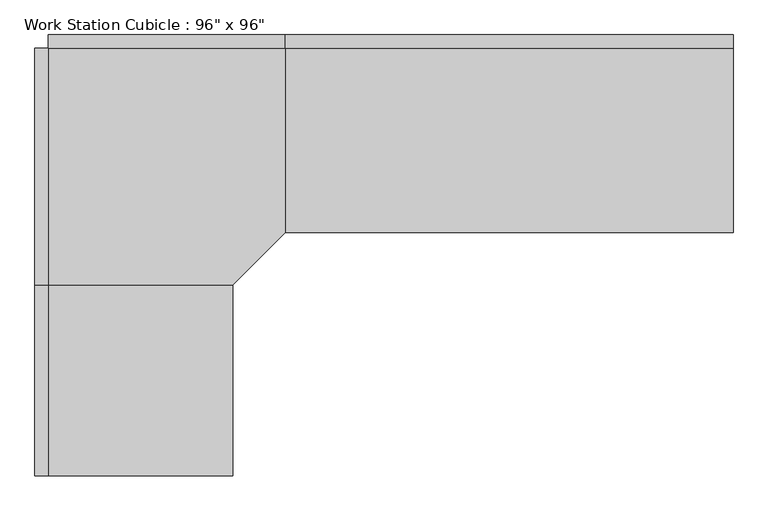
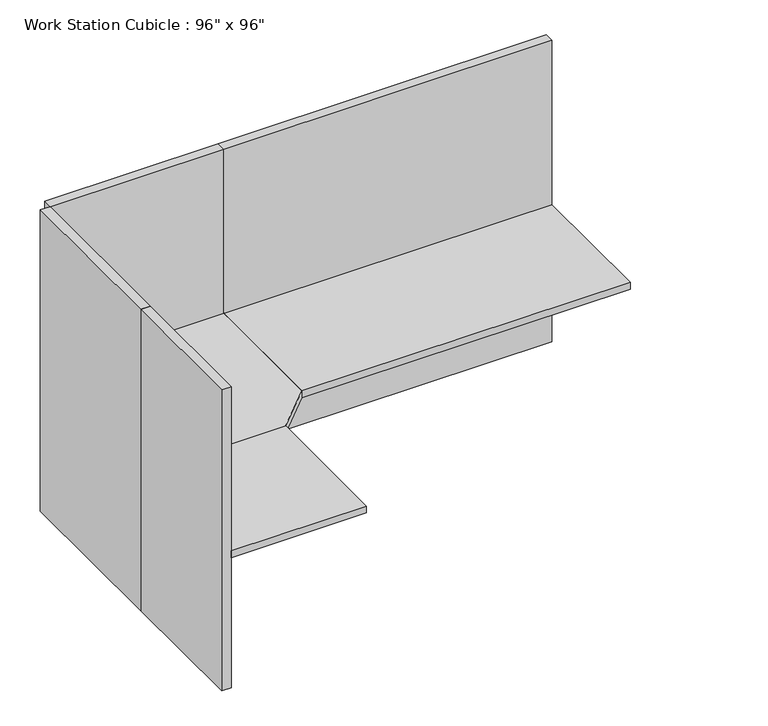
"""IFC4 building model written with IfcOpenShell, lengths in millimetres: furniture geometry."""

from ifc_helpers import new_model, si_unit, frame, origin, origin_with_axes, place, context, project, spatial, polyline, outline, extrude, source, transform, mapped, element, save


def furniture_c625fdf3(model_context):
    return source(origin(), model_context, "Body", "SweptSolid", [
        extrude(outline(polyline([(-80.9317522, -545.8230076), (833.4682478, -545.8230076), (833.4682478, -1257.0230076), (630.2682478, -1460.2230076), (-80.9317522, -1460.2230076), (-80.9317522, -545.8230076)])), frame((0.0, 0.0, 723.9), z_axis=(0.0, 0.0, 1.0), x_axis=(1.0, 0.0, 0.0)), (0.0, 0.0, 1.0), 38.1),
        extrude(outline(polyline([(630.2682478, -2196.8230076), (-80.9317522, -2196.8230076), (-80.9317522, -1460.2230076), (630.2682478, -1460.2230076), (630.2682478, -2196.8230076)])), frame((0.0, 0.0, 723.9), z_axis=(0.0, 0.0, 1.0), x_axis=(1.0, 0.0, 0.0)), (0.0, 0.0, 1.0), 38.1),
        extrude(outline(polyline([(2560.6682478, -1257.0230076), (833.4682478, -1257.0230076), (833.4682478, -545.8230076), (2560.6682478, -545.8230076), (2560.6682478, -1257.0230076)])), frame((0.0, 0.0, 723.9), z_axis=(0.0, 0.0, 1.0), x_axis=(1.0, 0.0, 0.0)), (0.0, 0.0, 1.0), 38.1),
        extrude(outline(polyline([(2560.6682478, -545.8230076), (833.4682478, -545.8230076), (833.4682478, -495.0230076), (2560.6682478, -495.0230076), (2560.6682478, -545.8230076)])), origin_with_axes(), (0.0, 0.0, 1.0), 1676.4),
        extrude(outline(polyline([(833.4682478, -545.8230076), (-80.9317522, -545.8230076), (-80.9317522, -495.0230076), (833.4682478, -495.0230076), (833.4682478, -545.8230076)])), origin_with_axes(), (0.0, 0.0, 1.0), 1676.4),
        extrude(outline(polyline([(-80.9317522, -1460.2230076), (-131.7317522, -1460.2230076), (-131.7317522, -545.8230076), (-80.9317522, -545.8230076), (-80.9317522, -1460.2230076)])), origin_with_axes(), (0.0, 0.0, 1.0), 1676.4),
        extrude(outline(polyline([(-80.9317522, -2196.8230076), (-131.7317522, -2196.8230076), (-131.7317522, -1460.2230076), (-80.9317522, -1460.2230076), (-80.9317522, -2196.8230076)])), origin_with_axes(), (0.0, 0.0, 1.0), 1676.4),
    ])


if __name__ == "__main__":
    model = new_model("IFC4")
    model_context = context("Model", 3, world=origin())
    ifc_project = project(units=[si_unit("LENGTHUNIT", "METRE", prefix="MILLI")], contexts=[model_context])
    site = spatial("IfcSite", under=ifc_project)
    building = spatial("IfcBuilding", under=site)
    placement = place(None, origin())
    furniture_shape = furniture_c625fdf3(model_context)
    element("IfcFurniture", 1, ObjectType="Work Station Cubicle : 96\" x 96\"", at=placement, inside=building, context=model_context, shape_type="MappedRepresentation", body=[
        mapped(furniture_shape, transform((0.0, 0.0, 0.0), x_axis=(1.0, 0.0, 0.0), y_axis=(0.0, 1.0, 0.0), z_axis=(0.0, 0.0, 1.0))),
    ])
    save(model, "model.ifc")

# Revit data of these elements
# Type "Work Station Cubicle : 96\" x 96\""
#   Assembly Code = "E2020"
#   Desktop Height = 2' - 6"
#   Desktop1 Width = 2' - 4"
#   Desktop2 Width = 2' - 4"
#   Panel Height = 5' - 6"
#   Panel1 Length = 2' - 5"
#   Panel2 Length = 5' - 8"
#   Cube Panel Material = Textile - Light Gray
#   Work Top Material = Laminate, Ivory, Matte
#   Default Elevation = 0
# Element 1 (IfcFurniture, "Work Station Cubicle : 96\" x 96\"")
#   Materials on its faces: "Textile - Light Gray", "Laminate, Ivory, Matte"
# Materials
#   "Textile - Light Gray": class "Fabric", colour RGB 204 204 204, transparency 0
#   "Laminate, Ivory, Matte": class "Plastic", colour RGB 247 247 239, transparency 0, Description = "Plastic Laminate - Ivory, Matte", Cost = 0
